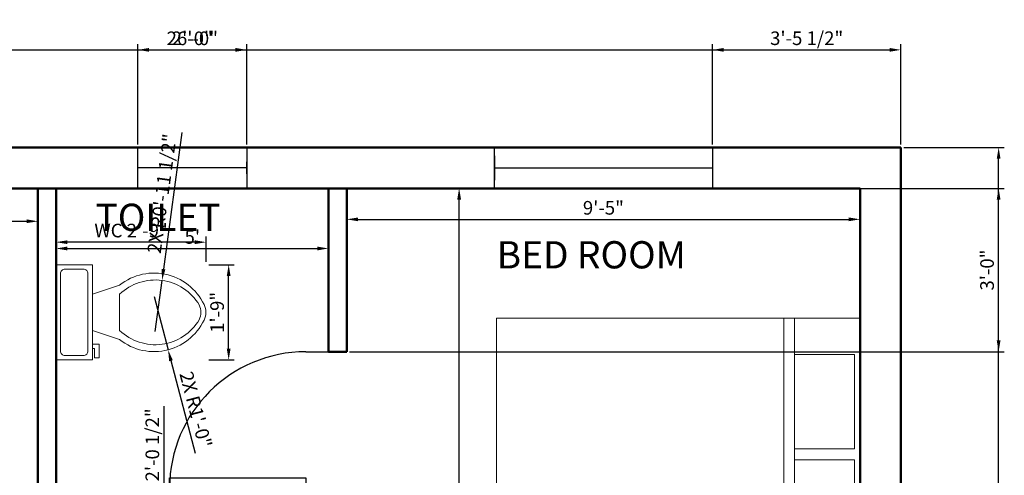
# Model space of a CAD drawing. Units: inches. Extents: x 1767 to 2185, y 3382 to 3854.
# Tile 4 of 4: x 1950 to 2167, y 3754 to 3854. Entities that reach past the tile are written whole.
import ezdxf

# ---------------------------------------------------------------- set-up
doc = ezdxf.new("R2010")
doc.units = ezdxf.units.IN
for name, color, linetype, lineweight in [('A-ANNO-DIMS', 2, 'Continuous', 18), ('A-AREA-IDEN', 7, 'Continuous', 25), ('A-DOOR', 3, 'Continuous', 25), ('A-FLOR-FIXT', 9, 'Continuous', 20), ('A-FURN', 8, 'Continuous', 18), ('A-GLAZ', 4, 'Continuous', 25), ('A-WALL', 7, 'Continuous', 50)]:
    doc.layers.add(name, color=color, linetype=linetype, lineweight=lineweight)
doc.styles.get("Standard").update_dxf_attribs({"font": 'arial.ttf'})
doc.dimstyles.new('ISO-25', dxfattribs={"dimtxt": 3, "dimasz": 2.5, "dimexe": 1.25, "dimexo": 0.625, "dimtad": 1, "dimdec": 0, "dimlunit": 3, "dimtxsty": 'Standard', "dimcen": 2.5, "dimadec": 0, "dimazin": 0, "dimtfac": 1, "dimtdec": 0, "dimtmove": 0, "dimatfit": 3, "dimfxl": 1, "dimarcsym": 0})

# ---------------------------------------------------------------- blocks, each defined once
blk = doc.blocks.new('*U2')
for p, q in [((0, 0), (0, -100)), ((600, 0), (600, -100))]:
    blk.add_line(p, q)
blk.add_lwpolyline([(0, 0), (0, 600), (43.75, 600), (43.75, 0)], close=True)
blk.add_arc((0, 0), 600, 0, 90)
blk = doc.blocks.new('*U4')
for p, q in [((0, 100), (0, 0)), ((900, 100), (900, 0)), ((0, 50), (900, 50))]:
    blk.add_line(p, q)
blk = doc.blocks.new('Toilet - top')
for p, q in [((9.5, -6), (9.5, -2)), ((-10, -8.5), (-8, -8.5)), ((-10, -9.5), (-10, -8.5)), ((-8, -8.5), (-8, -8)), ((-7, -8), (-7, -9.5)), ((-4, -8), (-6, -14)), ((4, -8), (6, -14)), ((-7, -9.5), (-10, -9.5)), ((4, -14), (-4, -14))]:
    blk.add_line(p, q)
blk.add_lwpolyline([(10.5, -8), (10.5, 0), (-10.5, 0), (-10.5, -8)], close=True)
for points in [[(-9.5, -2), (-9.5, -6)], [(8.5, -1), (-8.5, -1)], [(-8.5, -7), (8.5, -7)]]:
    blk.add_lwpolyline(points)
for centre, radius, start, end in [((-8.62, -1.88), 0.884, 81.8699, 188.1301), ((8.62, -1.88), 0.884, 351.8699, 98.1301), ((-8.62, -6.12), 0.884, 171.8699, 278.1301), ((8.62, -6.12), 0.884, 261.8699, 8.1301), ((3.52, -21.58), 12.17, 141.4691, 247.9714), ((4.2, -21.82), 11.33, 136.3677, 238.9468), ((-3.52, -21.58), 12.17, 292.0284, 38.5307), ((-4.2, -21.82), 11.33, 301.053, 43.6321), ((0, -27.88), 4, 245.7318, 294.2682), ((0, -29), 4, 254.8605, 285.1395)]:
    blk.add_arc(centre, radius, start, end)
blk = doc.blocks.new('Bed - Queen')
for p, q in [((0, -80.00003), (0, 0)), ((0, 0), (59.99999, 0)), ((59.99999, 0), (59.99999, -80.00003)), ((7.99999, -1.2), (28.79998, -1.2)), ((7.99999, -14.4), (7.99999, -1.2)), ((28.79998, -1.2), (28.79998, -14.4)), ((31.19999, -1.2), (51.99999, -1.2)), ((31.19999, -14.4), (31.19999, -1.2)), ((51.99999, -1.2), (51.99999, -16.4)), ((0, -14.4), (44.8, -14.4)), ((59.99999, -29.6), (44.8, -14.4)), ((44.8, -14.4), (44.8, -29.6)), ((44.8, -16.8), (0, -16.8)), ((51.99999, -16.4), (46.79936, -16.4)), ((44.8, -29.6), (59.99999, -29.6)), ((59.99999, -80.00003), (0, -80.00003))]:
    blk.add_line(p, q)
blk = doc.blocks.new('*D10')
at = {"layer": 'A-ANNO-DIMS', "color": 0, "lineweight": -2, "transparency": 16777216}
for p, q in [((1841.16, 3816.53), (1841.16, 3808.64)), ((1954.16, 3816.53), (1954.16, 3808.64)), ((1843.66, 3809.89), (1951.66, 3809.89))]:
    blk.add_line(p, q, dxfattribs=at)
at = {"layer": 'A-ANNO-DIMS', "color": 0, "transparency": 16777216}
for points in [[(1843.66, 3810.31), (1843.66, 3809.48), (1841.16, 3809.89)], [(1951.66, 3810.31), (1951.66, 3809.48), (1954.16, 3809.89)]]:
    blk.add_solid(points, dxfattribs=at)
at = {"layer": 'Defpoints', "color": 0, "transparency": 16777216}
for p in [(1841.16, 3817.15), (1954.16, 3817.15), (1954.16, 3809.89)]:
    blk.add_point(p, dxfattribs=at)
at = {"layer": 'A-ANNO-DIMS', "color": 0, "transparency": 16777216, "insert": (1897.66, 3812.05), "char_height": 3, "attachment_point": 5}
blk.add_mtext('9\'-5"', dxfattribs=at)
blk = doc.blocks.new('*D12')
at = {"layer": 'A-ANNO-DIMS', "color": 0, "lineweight": -2, "transparency": 16777216}
for p, q in [((2022.16, 3816.53), (2022.16, 3809.07)), ((2135.16, 3816.53), (2135.16, 3809.07)), ((2024.66, 3810.32), (2132.66, 3810.32))]:
    blk.add_line(p, q, dxfattribs=at)
at = {"layer": 'A-ANNO-DIMS', "color": 0, "transparency": 16777216}
for points in [[(2024.66, 3810.73), (2024.66, 3809.9), (2022.16, 3810.32)], [(2132.66, 3810.73), (2132.66, 3809.9), (2135.16, 3810.32)]]:
    blk.add_solid(points, dxfattribs=at)
at = {"layer": 'Defpoints', "color": 0, "transparency": 16777216}
for p in [(2022.16, 3817.15), (2135.16, 3817.15), (2135.16, 3810.32)]:
    blk.add_point(p, dxfattribs=at)
at = {"layer": 'A-ANNO-DIMS', "color": 0, "transparency": 16777216, "insert": (2078.66, 3812.47), "char_height": 3, "attachment_point": 5}
blk.add_mtext('9\'-5"', dxfattribs=at)
blk = doc.blocks.new('*D13')
at = {"layer": 'A-ANNO-DIMS', "color": 0, "lineweight": -2, "transparency": 16777216}
for p, q in [((2134.53, 3817.15), (2045.65, 3817.15)), ((2046.9, 3675.65), (2046.9, 3814.65)), ((2134.53, 3673.15), (2045.65, 3673.15))]:
    blk.add_line(p, q, dxfattribs=at)
at = {"layer": 'A-ANNO-DIMS', "color": 0, "transparency": 16777216}
for points in [[(2046.48, 3814.65), (2047.32, 3814.65), (2046.9, 3817.15)], [(2046.48, 3675.65), (2047.32, 3675.65), (2046.9, 3673.15)]]:
    blk.add_solid(points, dxfattribs=at)
at = {"layer": 'Defpoints', "color": 0, "transparency": 16777216}
for p in [(2046.9, 3817.15), (2135.16, 3817.15), (2135.16, 3673.15)]:
    blk.add_point(p, dxfattribs=at)
at = {"layer": 'A-ANNO-DIMS', "color": 0, "transparency": 16777216, "insert": (2044.77, 3745.15), "char_height": 3, "attachment_point": 5, "rotation": 90}
blk.add_mtext("12'", dxfattribs=at)
blk = doc.blocks.new('*D14')
at = {"layer": 'A-ANNO-DIMS', "color": 0, "lineweight": -2, "transparency": 16777216}
for p, q in [((1958.16, 3816.53), (1958.16, 3802.65)), ((2018.16, 3816.53), (2018.16, 3802.65)), ((1960.66, 3803.9), (2015.66, 3803.9))]:
    blk.add_line(p, q, dxfattribs=at)
at = {"layer": 'A-ANNO-DIMS', "color": 0, "transparency": 16777216}
for points in [[(1960.66, 3804.32), (1960.66, 3803.48), (1958.16, 3803.9)], [(2015.66, 3804.32), (2015.66, 3803.48), (2018.16, 3803.9)]]:
    blk.add_solid(points, dxfattribs=at)
at = {"layer": 'Defpoints', "color": 0, "transparency": 16777216}
for p in [(1958.16, 3817.15), (2018.16, 3817.15), (2018.16, 3803.9)]:
    blk.add_point(p, dxfattribs=at)
at = {"layer": 'A-ANNO-DIMS', "color": 0, "transparency": 16777216, "insert": (1988.16, 3806.05), "char_height": 3, "attachment_point": 5}
blk.add_mtext("5'", dxfattribs=at)
blk = doc.blocks.new('*D33')
at = {"layer": 'A-ANNO-DIMS', "color": 0, "lineweight": -2, "transparency": 16777216}
for p, q in [((1958.16, 3800.95), (1958.16, 3806.54)), ((1991.21, 3800.95), (1991.21, 3806.54)), ((1988.71, 3805.29), (1960.66, 3805.29))]:
    blk.add_line(p, q, dxfattribs=at)
at = {"layer": 'A-ANNO-DIMS', "color": 0, "transparency": 16777216}
for points in [[(1960.66, 3805.7), (1960.66, 3804.87), (1958.16, 3805.29)], [(1988.71, 3805.7), (1988.71, 3804.87), (1991.21, 3805.29)]]:
    blk.add_solid(points, dxfattribs=at)
at = {"layer": 'Defpoints', "color": 0, "transparency": 16777216}
for p in [(1958.16, 3805.29), (1958.16, 3800.33), (1991.21, 3800.33)]:
    blk.add_point(p, dxfattribs=at)
at = {"layer": 'A-ANNO-DIMS', "color": 0, "transparency": 16777216, "insert": (1974.68, 3807.46), "char_height": 3, "attachment_point": 5}
blk.add_mtext('WC 2\'-9"', dxfattribs=at)
blk = doc.blocks.new('*D34')
at = {"layer": 'A-ANNO-DIMS', "color": 0, "lineweight": -2, "transparency": 16777216}
for p, q in [((1991.83, 3800.33), (1997.41, 3800.33)), ((1996.16, 3781.83), (1996.16, 3797.83)), ((1991.83, 3779.33), (1997.41, 3779.33))]:
    blk.add_line(p, q, dxfattribs=at)
at = {"layer": 'A-ANNO-DIMS', "color": 0, "transparency": 16777216}
for points in [[(1995.75, 3797.83), (1996.58, 3797.83), (1996.16, 3800.33)], [(1995.75, 3781.83), (1996.58, 3781.83), (1996.16, 3779.33)]]:
    blk.add_solid(points, dxfattribs=at)
at = {"layer": 'Defpoints', "color": 0, "transparency": 16777216}
for p in [(1991.21, 3800.33), (1996.16, 3800.33), (1991.21, 3779.33)]:
    blk.add_point(p, dxfattribs=at)
at = {"layer": 'A-ANNO-DIMS', "color": 0, "transparency": 16777216, "insert": (1994.01, 3789.83), "char_height": 3, "attachment_point": 5, "rotation": 90}
blk.add_mtext('1\'-9"', dxfattribs=at)
blk = doc.blocks.new('*D35')
at = {"layer": 'A-ANNO-DIMS', "color": 0, "lineweight": -2, "transparency": 16777216}
for p, q in [((1981.93, 3736.86), (1981.93, 3769.19)), ((1978.87, 3736.86), (1983.18, 3736.86)), ((1981.93, 3714.81), (1981.93, 3734.36)), ((1978.87, 3712.31), (1983.18, 3712.31))]:
    blk.add_line(p, q, dxfattribs=at)
at = {"layer": 'A-ANNO-DIMS', "color": 0, "transparency": 16777216}
for points in [[(1981.51, 3734.36), (1982.34, 3734.36), (1981.93, 3736.86)], [(1981.51, 3714.81), (1982.34, 3714.81), (1981.93, 3712.31)]]:
    blk.add_solid(points, dxfattribs=at)
at = {"layer": 'Defpoints', "color": 0, "transparency": 16777216}
for p in [(1978.24, 3736.86), (1981.93, 3736.86), (1978.24, 3712.31)]:
    blk.add_point(p, dxfattribs=at)
at = {"layer": 'A-ANNO-DIMS', "color": 0, "transparency": 16777216, "insert": (1979.75, 3754.28), "char_height": 3, "attachment_point": 5, "rotation": 90}
blk.add_mtext('BASIN 2\'-0 1/2"', dxfattribs=at)
blk = doc.blocks.new('*D39')
at = {"layer": 'A-ANNO-DIMS', "color": 0, "lineweight": -2, "transparency": 16777216}
for p, q in [((1832.16, 3826.78), (1832.16, 3848.91)), ((1834.66, 3847.66), (2141.66, 3847.66)), ((2144.16, 3826.78), (2144.16, 3848.91))]:
    blk.add_line(p, q, dxfattribs=at)
at = {"layer": 'A-ANNO-DIMS', "color": 0, "transparency": 16777216}
for points in [[(1834.66, 3848.07), (1834.66, 3847.24), (1832.16, 3847.66)], [(2141.66, 3848.07), (2141.66, 3847.24), (2144.16, 3847.66)]]:
    blk.add_solid(points, dxfattribs=at)
at = {"layer": 'Defpoints', "color": 0, "transparency": 16777216}
for p in [(2144.16, 3847.66), (1832.16, 3826.15), (2144.16, 3826.15)]:
    blk.add_point(p, dxfattribs=at)
at = {"layer": 'A-ANNO-DIMS', "color": 0, "transparency": 16777216, "insert": (1988.16, 3849.81), "char_height": 3, "attachment_point": 5}
blk.add_mtext('26\'-0"', dxfattribs=at)
blk = doc.blocks.new('*D40')
at = {"layer": 'A-ANNO-DIMS', "color": 0, "lineweight": -2, "transparency": 16777216}
for p, q in [((2144.78, 3826.15), (2166.91, 3826.15)), ((2165.66, 3408.65), (2165.66, 3823.65)), ((2144.78, 3406.15), (2166.91, 3406.15))]:
    blk.add_line(p, q, dxfattribs=at)
at = {"layer": 'A-ANNO-DIMS', "color": 0, "transparency": 16777216}
for points in [[(2165.25, 3823.65), (2166.08, 3823.65), (2165.66, 3826.15)], [(2165.25, 3408.65), (2166.08, 3408.65), (2165.66, 3406.15)]]:
    blk.add_solid(points, dxfattribs=at)
at = {"layer": 'Defpoints', "color": 0, "transparency": 16777216}
for p in [(2144.16, 3826.15), (2165.66, 3826.15), (2144.16, 3406.15)]:
    blk.add_point(p, dxfattribs=at)
at = {"layer": 'A-ANNO-DIMS', "color": 0, "transparency": 16777216, "insert": (2163.51, 3616.15), "char_height": 3, "attachment_point": 5, "rotation": 90}
blk.add_mtext('35\'-0"', dxfattribs=at)
blk = doc.blocks.new('*D44')
at = {"layer": 'A-ANNO-DIMS', "color": 0, "lineweight": -2, "transparency": 16777216}
for p, q in [((1976.16, 3826.78), (1976.16, 3848.91)), ((1978.66, 3847.66), (1997.66, 3847.66)), ((2000.16, 3826.78), (2000.16, 3848.91))]:
    blk.add_line(p, q, dxfattribs=at)
at = {"layer": 'A-ANNO-DIMS', "color": 0, "transparency": 16777216}
for points in [[(1978.66, 3848.07), (1978.66, 3847.24), (1976.16, 3847.66)], [(1997.66, 3848.07), (1997.66, 3847.24), (2000.16, 3847.66)]]:
    blk.add_solid(points, dxfattribs=at)
at = {"layer": 'Defpoints', "color": 0, "transparency": 16777216}
for p in [(2000.16, 3847.66), (1976.16, 3826.15), (2000.16, 3826.15)]:
    blk.add_point(p, dxfattribs=at)
at = {"layer": 'A-ANNO-DIMS', "color": 0, "transparency": 16777216, "insert": (1988.16, 3849.81), "char_height": 3, "attachment_point": 5}
blk.add_mtext('2\'-0"', dxfattribs=at)
blk = doc.blocks.new('*D46')
at = {"layer": 'A-ANNO-DIMS', "color": 0, "lineweight": -2, "transparency": 16777216}
for p, q in [((2102.66, 3826.78), (2102.66, 3848.91)), ((2105.16, 3847.66), (2141.66, 3847.66)), ((2144.16, 3826.78), (2144.16, 3848.91))]:
    blk.add_line(p, q, dxfattribs=at)
at = {"layer": 'A-ANNO-DIMS', "color": 0, "transparency": 16777216}
for points in [[(2105.16, 3848.07), (2105.16, 3847.24), (2102.66, 3847.66)], [(2141.66, 3848.07), (2141.66, 3847.24), (2144.16, 3847.66)]]:
    blk.add_solid(points, dxfattribs=at)
at = {"layer": 'Defpoints', "color": 0, "transparency": 16777216}
for p in [(2144.16, 3847.66), (2102.66, 3826.15), (2144.16, 3826.15)]:
    blk.add_point(p, dxfattribs=at)
at = {"layer": 'A-ANNO-DIMS', "color": 0, "transparency": 16777216, "insert": (2123.41, 3849.83), "char_height": 3, "attachment_point": 5}
blk.add_mtext('3\'-5 1/2"', dxfattribs=at)
blk = doc.blocks.new('*D50')
at = {"layer": 'A-ANNO-DIMS', "color": 0, "lineweight": -2, "transparency": 16777216}
for p, q in [((2022.78, 3817.15), (2166.91, 3817.15)), ((2165.66, 3783.65), (2165.66, 3814.65)), ((2022.78, 3781.15), (2166.91, 3781.15))]:
    blk.add_line(p, q, dxfattribs=at)
at = {"layer": 'A-ANNO-DIMS', "color": 0, "transparency": 16777216}
for points in [[(2165.25, 3814.65), (2166.08, 3814.65), (2165.66, 3817.15)], [(2165.25, 3783.65), (2166.08, 3783.65), (2165.66, 3781.15)]]:
    blk.add_solid(points, dxfattribs=at)
at = {"layer": 'Defpoints', "color": 0, "transparency": 16777216}
for p in [(2022.16, 3817.15), (2165.66, 3817.15), (2022.16, 3781.15)]:
    blk.add_point(p, dxfattribs=at)
at = {"layer": 'A-ANNO-DIMS', "color": 0, "transparency": 16777216, "insert": (2163.51, 3799.15), "char_height": 3, "attachment_point": 5, "rotation": 90}
blk.add_mtext('3\'-0"', dxfattribs=at)
blk = doc.blocks.new('*D53')
at = {"layer": 'A-ANNO-DIMS', "color": 0, "lineweight": -2, "transparency": 16777216}
for p, q in [((1979.74, 3793.35), (1982.83, 3781.58)), ((1988.83, 3758.76), (1983.47, 3779.16))]:
    blk.add_line(p, q, dxfattribs=at)
at = {"layer": 'A-ANNO-DIMS', "color": 0, "transparency": 16777216}
blk.add_solid([(1983.87, 3779.27), (1983.06, 3779.06), (1982.83, 3781.58)], dxfattribs=at)
at = {"layer": 'Defpoints', "color": 0, "transparency": 16777216}
for p in [(1979.74, 3793.35), (1982.83, 3781.58)]:
    blk.add_point(p, dxfattribs=at)
at = {"layer": 'A-ANNO-DIMS', "color": 0, "transparency": 16777216, "insert": (1988.55, 3768.3), "char_height": 3, "attachment_point": 5, "rotation": 284.7214}
blk.add_mtext('2X R1\'-0"', dxfattribs=at)
blk = doc.blocks.new('*D54')
at = {"layer": 'A-ANNO-DIMS', "color": 0, "lineweight": -2, "transparency": 16777216}
for p, q in [((1985.87, 3829.48), (1981.82, 3799.34)), ((1979.98, 3785.63), (1981.49, 3796.86))]:
    blk.add_line(p, q, dxfattribs=at)
at = {"layer": 'A-ANNO-DIMS', "color": 0, "transparency": 16777216}
blk.add_solid([(1981.41, 3799.39), (1982.23, 3799.28), (1981.49, 3796.86)], dxfattribs=at)
at = {"layer": 'Defpoints', "color": 0, "transparency": 16777216}
for p in [(1981.49, 3796.86), (1979.98, 3785.63)]:
    blk.add_point(p, dxfattribs=at)
at = {"layer": 'A-ANNO-DIMS', "color": 0, "transparency": 16777216, "insert": (1981.86, 3815.94), "char_height": 3, "attachment_point": 5, "rotation": 82.3432}
blk.add_mtext('2X R0\'-11 1/2"', dxfattribs=at)

msp = doc.modelspace()

# ---------------------------------------------------------------- linework, layer by layer
at = {"layer": 'A-GLAZ'}
for p, q in [((1976.16, 3817.15), (1976.16, 3826.15)), ((1976.16, 3826.15), (2000.16, 3826.15)), ((2000.16, 3826.15), (2000.16, 3817.15)), ((2054.66, 3817.15), (2054.66, 3826.15)), ((2054.66, 3826.15), (2102.66, 3826.15)), ((2102.66, 3826.15), (2102.66, 3817.15)), ((2102.66, 3817.15), (2054.66, 3817.15))]:
    msp.add_line(p, q, dxfattribs=at)
at = {"layer": 'A-WALL'}
for p, q in [((1832.16, 3826.15), (2144.16, 3826.15)), ((2144.16, 3826.15), (2144.16, 3406.15)), ((1841.16, 3817.15), (2135.16, 3817.15)), ((1954.16, 3669.15), (1954.16, 3817.15)), ((1958.16, 3669.15), (1958.16, 3817.15)), ((2018.16, 3817.15), (2018.16, 3781.15)), ((2022.16, 3817.15), (2022.16, 3781.15)), ((2135.16, 3817.15), (2135.16, 3415.15)), ((2018.16, 3781.15), (2022.16, 3781.15))]:
    msp.add_line(p, q, dxfattribs=at)

# ---------------------------------------------------------------- block references
at = {"layer": 'A-DOOR', "xscale": 0.0500000000000001, "yscale": 0.0500000000000001, "zscale": 0.0500000000000001, "rotation": 90}
msp.add_blockref('*U2', (2013.16, 3751.15), dxfattribs=at)
at = {"layer": 'A-FLOR-FIXT', "rotation": 90}
msp.add_blockref('Toilet - top', (1958.16, 3789.83), dxfattribs=at)
at = {"layer": 'A-FURN', "rotation": 269.9999999999998}
msp.add_blockref('Bed - Queen', (2135.16, 3788.57), dxfattribs=at)
at = {"layer": 'A-GLAZ', "xscale": 0.0533333333333335, "yscale": 0.0533333333333335, "zscale": 0.0533333333333335}
msp.add_blockref('*U4', (2054.66, 3818.98), dxfattribs=at)
at = {"layer": 'A-GLAZ', "xscale": 0.0266666666666666, "yscale": 0.0266666666666666, "zscale": 0.0266666666666666, "rotation": 180}
msp.add_blockref('*U4', (2000.16, 3822.98), dxfattribs=at)

# ---------------------------------------------------------------- texts
at = {"layer": 'A-AREA-IDEN'}
for s, p in [('TOILET', (1966.85, 3807.77)), ('BED ROOM', (2055.16, 3799.51))]:
    msp.add_text(s, height=6, dxfattribs=at).set_placement(p)

# ---------------------------------------------------------------- dimensions: what is measured, and where the dimension line sits
at = {"layer": 'A-ANNO-DIMS'}
for base, p1, p2, override, picture, middle in [((2144.16, 3847.66), (2102.66, 3826.15), (2144.16, 3826.15), {"dimdec": 1, "dimlfac": 1, "dimrnd": 0, "dimzin": 1, "dimdsep": 46, "dimlunit": 4, "dimfrac": 2}, '*D46', (2123.41, 3849.83)), ((2144.16, 3847.66), (1832.16, 3826.15), (2144.16, 3826.15), {"dimdec": 1, "dimlfac": 1, "dimrnd": 0, "dimzin": 1, "dimdsep": 46, "dimlunit": 4, "dimfrac": 2}, '*D39', (1988.16, 3849.81)), ((2000.16, 3847.66), (1976.16, 3826.15), (2000.16, 3826.15), {"dimdec": 1, "dimlfac": 1, "dimrnd": 0, "dimzin": 1, "dimdsep": 46, "dimlunit": 4, "dimfrac": 2}, '*D44', (1988.16, 3849.81)), ((1954.16, 3809.89), (1841.16, 3817.15), (1954.16, 3817.15), {"dimclrd": 0, "dimclre": 0, "dimclrt": 0}, '*D10', (1897.66, 3812.05)), ((2018.16, 3803.9), (1958.16, 3817.15), (2018.16, 3817.15), {"dimclrd": 0, "dimclre": 0, "dimclrt": 0}, '*D14', (1988.16, 3806.05)), ((2135.16, 3810.32), (2022.16, 3817.15), (2135.16, 3817.15), {"dimclrd": 0, "dimclre": 0, "dimclrt": 0}, '*D12', (2078.66, 3812.47))]:
    dim = msp.add_linear_dim(base=base, p1=p1, p2=p2, dimstyle='ISO-25', override=override, dxfattribs=at)
    dim.commit()
    dim.dimension.update_dxf_attribs({"geometry": picture, "text_midpoint": middle})
for center, mpoint, picture, middle in [((1979.98, 3785.63), (1981.49, 3796.86), '*D54', (1981.86, 3815.94)), ((1979.74, 3793.35), (1982.83, 3781.58), '*D53', (1988.55, 3768.3))]:
    dim = msp.add_radius_dim(center=center, mpoint=mpoint, text='2X <>', dimstyle='ISO-25', override={"dimdec": 1, "dimlfac": 1, "dimrnd": 0, "dimzin": 1, "dimdsep": 46, "dimlunit": 4, "dimfrac": 2}, dxfattribs=at)
    dim.commit()
    dim.dimension.update_dxf_attribs({"geometry": picture, "text_midpoint": middle})
for base, p1, p2, override, picture, middle in [((2165.66, 3826.15), (2144.16, 3406.15), (2144.16, 3826.15), {"dimdec": 1, "dimlfac": 1, "dimrnd": 0, "dimzin": 1, "dimdsep": 46, "dimlunit": 4, "dimfrac": 2}, '*D40', (2163.51, 3616.15)), ((2165.66, 3817.15), (2022.16, 3781.15), (2022.16, 3817.15), {"dimdec": 1, "dimlfac": 1, "dimrnd": 0, "dimzin": 1, "dimdsep": 46, "dimlunit": 4, "dimfrac": 2}, '*D50', (2163.51, 3799.15)), ((2046.9, 3817.15), (2135.16, 3673.15), (2135.16, 3817.15), {"dimclrd": 0, "dimclre": 0, "dimclrt": 0}, '*D13', (2044.77, 3745.15)), ((1996.16, 3800.33), (1991.21, 3779.33), (1991.21, 3800.33), {"dimdec": 1, "dimlfac": 1, "dimrnd": 0, "dimzin": 1, "dimdsep": 46, "dimlunit": 4, "dimfrac": 2}, '*D34', (1994.01, 3789.83))]:
    dim = msp.add_linear_dim(base=base, p1=p1, p2=p2, angle=90, dimstyle='ISO-25', override=override, dxfattribs=at)
    dim.commit()
    dim.dimension.update_dxf_attribs({"geometry": picture, "text_midpoint": middle})
for base, p1, p2, angle, text, picture, middle in [((1958.1591, 3805.2869), (1991.2054, 3800.3299), (1958.1591, 3800.3299), 180, 'WC <>', '*D33', (1974.6823, 3807.463)), ((1981.9259, 3736.8648), (1978.2433, 3712.3139), (1978.2433, 3736.8648), 90, 'BASIN <>', '*D35', (1979.7498, 3754.2766))]:
    dim = msp.add_linear_dim(base=base, p1=p1, p2=p2, angle=angle, text=text, dimstyle='ISO-25', override={"dimdec": 1, "dimlfac": 1, "dimrnd": 0, "dimzin": 1, "dimdsep": 46, "dimlunit": 4, "dimfrac": 2}, dxfattribs=at)
    dim.commit()
    dim.dimension.update_dxf_attribs({"geometry": picture, "text_midpoint": middle})

doc.saveas('drawing.dxf')
